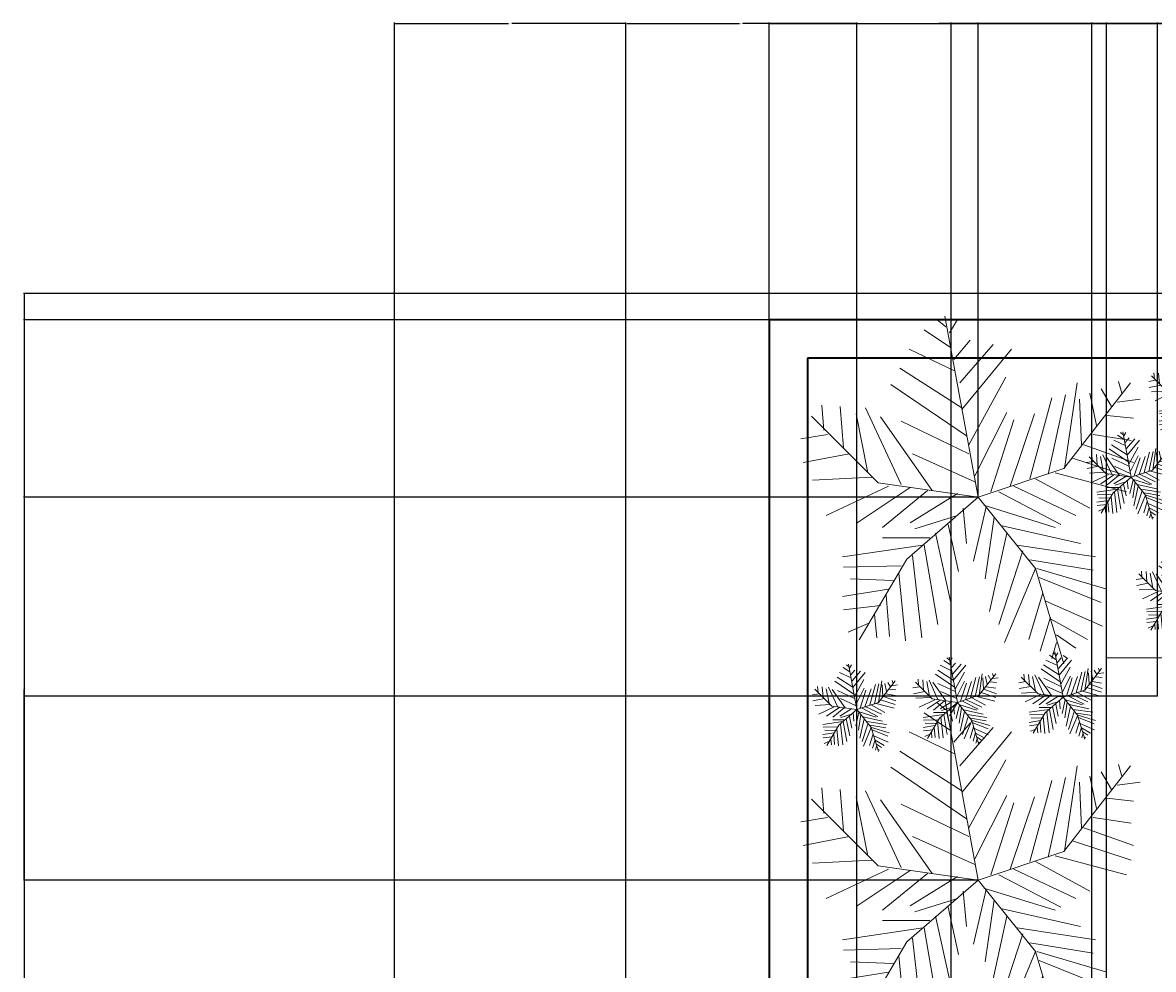
# Model space of a CAD drawing. Units: inches. Extents: x 818 to 1898, y 976 to 2364.
# Tile 61 of 96: x 818 to 1083, y 2142 to 2364. Entities that reach past the tile are written whole.
import ezdxf

# ---------------------------------------------------------------- set-up
doc = ezdxf.new("R2010")
doc.units = ezdxf.units.IN
doc.header["$LTSCALE"] = 5
doc.header["$MEASUREMENT"] = 0
for name, color, linetype, lineweight in [('A-ANNO-DIMS', 2, 'Continuous', 18), ('C-PROP', 7, 'Continuous', 35), ('L-PLNT-BEDS', 94, 'Continuous', 18)]:
    doc.layers.add(name, color=color, linetype=linetype, lineweight=lineweight)
doc.layers.add('L-PLNT', color=116, linetype='Continuous', lineweight=13, true_color=0x136734)
doc.styles.get("Standard").update_dxf_attribs({"font": 'arial.ttf'})
doc.dimstyles.get("Standard").update_dxf_attribs({"dimtxt": 0.18, "dimasz": 0.18, "dimexe": 0.18, "dimexo": 0.0625, "dimgap": 0.09, "dimtad": 0, "dimtih": 1, "dimtoh": 1, "dimdec": 4, "dimzin": 0, "dimdsep": 46, "dimtxsty": 'Standard', "dimcen": 0.09, "dimadec": 0, "dimazin": 0, "dimtfac": 1, "dimtdec": 4, "dimtofl": 0, "dimtmove": 0, "dimatfit": 3, "dimfxl": 1, "dimtolj": 1, "dimtzin": 0, "dimarcsym": 0})

# ---------------------------------------------------------------- blocks, each defined once
blk = doc.blocks.new('SHRUB-ACCENT')
for p, q in [((8.8, 18.63), (7.25, 19.67)), ((8.53, 19.84), (7.99, 20.28)), ((10.44, 9.82), (8.47, 20.47)), ((8.74, 19.5), (9.21, 20.28)), ((9.01, 17.93), (9.96, 19.06)), ((9.35, 16.54), (11.31, 18.8)), ((9.75, 13.42), (5.28, 16.46)), ((9.48, 15.07), (5.82, 17.41)), ((9.08, 17.24), (6.37, 18.54)), ((9.48, 14.98), (12.39, 18.54)), ((9.89, 12.9), (12.06, 16.89)), ((15.49, 11.5), (19.41, 16.55)), ((15.51, 11.51), (16.25, 16.54)), ((17, 15.94), (17.41, 14.03)), ((17.68, 16.2), (18.29, 15.16)), ((18.69, 16.63), (18.9, 15.94)), ((1.56, 13.51), (0, 13.25)), ((4.55, 10.66), (0.62, 14.58)), ((1.35, 13.77), (1.22, 15.24)), ((2.3, 15.16), (2.51, 12.72)), ((3.25, 14.72), (3.93, 11.25)), ((3.79, 15.07), (5.89, 10.55)), ((7.72, 10.21), (4.67, 14.55)), ((5.89, 14.29), (9.89, 12.38)), ((10.23, 11.07), (12.12, 14.81)), ((11.17, 10.12), (12.53, 14.37)), ((12.33, 10.47), (13.75, 14.72)), ((13.48, 10.9), (14.76, 15.68)), ((14.56, 11.16), (15.58, 15.85)), ((16.39, 15.59), (16.53, 12.9)), ((17.2, 13.51), (19.44, 13.16)), ((18.02, 14.63), (19.57, 14.46)), ((18.62, 15.42), (19.98, 15.59)), ((2.84, 12.38), (0.14, 11.86)), ((4.2, 10.99), (0.68, 10.81)), ((10.44, 9.82), (4.55, 10.66)), ((6.57, 12.38), (10.23, 10.73)), ((10.44, 9.82), (15.49, 11.5)), ((13.82, 10.9), (17, 9.16)), ((14.97, 11.25), (19.17, 10.12)), ((15.98, 12.12), (19.44, 10.99)), ((16.66, 12.9), (19.57, 11.86)), ((5.15, 10.47), (1.49, 8.73)), ((6.43, 10.38), (3.32, 8.3)), ((7.45, 10.21), (4.81, 8.04)), ((10.44, 9.82), (6.23, 6.17)), ((9.21, 10.03), (6.43, 8.3)), ((9.21, 8.73), (6.7, 7.95)), ((8.67, 8.21), (9.28, 5.43)), ((9.55, 9.16), (9.75, 7.08)), ((10.9, 9.25), (10.16, 6.04)), ((10.44, 9.82), (13.8, 5.61)), ((10.77, 9.34), (14.97, 8.04)), ((11.38, 8.64), (10.84, 5)), ((11.65, 10.12), (15.31, 8.21)), ((11.85, 8.12), (16.46, 7.08)), ((12.53, 10.47), (16.19, 8.73)), ((7.18, 6.99), (2.44, 6.3)), ((5.89, 5.78), (2.51, 5.69)), ((6.23, 6.17), (3.43, 1.4)), ((7.59, 7.43), (4.81, 7.43)), ((5.76, 5.34), (6.16, 1.35)), ((6.57, 6.39), (7.11, 1.52)), ((7.25, 6.99), (8.06, 2.31)), ((7.92, 7.69), (8.8, 3.69)), ((12.12, 7.69), (11.11, 3.09)), ((13.07, 6.65), (11.65, 2.31)), ((13.82, 5.6), (11.99, 1.26)), ((12.73, 6.99), (17.34, 6.3)), ((13.48, 6.13), (17.2, 5.52)), ((13.8, 5.61), (15.49, 0)), ((13.88, 5.6), (18.02, 4.39)), ((5.15, 4.39), (2.44, 3.95)), ((4.67, 3.43), (2.51, 3.17)), ((5.42, 4.91), (2.91, 5)), ((4.33, 2.91), (4.47, 1.52)), ((5.01, 4.04), (5.21, 1.61)), ((14.22, 4.13), (13.41, 1.44)), ((14.02, 5.08), (17.68, 3.61)), ((14.7, 2.74), (14.09, 0.74)), ((14.43, 3.69), (17.74, 2.22)), ((14.7, 2.65), (16.86, 1.44)), ((4, 2.39), (2.78, 1.87)), ((15.04, 1.26), (14.76, 0.31)), ((15.04, 1.7), (16.19, 0.92)), ((15.44, 0.48), (15.71, 0.31))]:
    blk.add_line(p, q)
blk = doc.blocks.new('PALM-BORDER')
for p, q in [((33.95, 78.95), (31.8, 80.68)), ((41.53, 39.05), (33.72, 81.45)), ((34.76, 77.57), (36.65, 80.68)), ((35.03, 74.11), (28.83, 78.26)), ((35.84, 71.35), (39.61, 75.84)), ((37.18, 65.82), (45, 74.8)), ((36.11, 68.59), (25.33, 73.77)), ((37.72, 59.6), (49.31, 73.77)), ((37.72, 59.95), (23.17, 69.28)), ((39.34, 51.31), (47.96, 67.2)), ((38.8, 53.39), (21.02, 65.48)), ((61.61, 45.75), (77.23, 65.83)), ((61.71, 45.79), (64.67, 65.82)), ((70.33, 64.44), (72.75, 60.3)), ((74.37, 66.17), (75.18, 63.4)), ((53.62, 43.37), (58.74, 62.37)), ((57.93, 44.41), (61.97, 63.06)), ((65.21, 62.02), (65.75, 51.31)), ((67.63, 63.4), (69.25, 55.81)), ((74.1, 61.33), (79.49, 62.02)), ((5.39, 54.77), (4.85, 60.64)), ((9.16, 60.3), (9.97, 50.62)), ((12.93, 58.57), (15.63, 44.75)), ((15.09, 59.95), (23.44, 41.99)), ((40.69, 44.06), (48.23, 58.91)), ((49.04, 41.64), (54.7, 58.57)), ((18.1, 42.4), (2.48, 58.02)), ((30.72, 40.61), (18.59, 57.88)), ((23.44, 56.84), (39.34, 49.24)), ((44.46, 40.26), (49.85, 57.19)), ((71.68, 58.22), (77.87, 57.53)), ((6.2, 53.73), (0, 52.7)), ((68.44, 53.73), (77.33, 52.35)), ((66.29, 51.31), (77.87, 47.17)), ((11.32, 49.24), (0.54, 47.17)), ((26.14, 49.24), (40.69, 42.68)), ((63.59, 48.21), (77.33, 43.71)), ((41.53, 39.05), (61.61, 45.75)), ((16.71, 43.71), (2.69, 43.02)), ((41.53, 39.05), (18.1, 42.4)), ((54.97, 43.37), (67.63, 36.46)), ((59.55, 44.75), (76.26, 40.26)), ((20.48, 41.64), (5.93, 34.73)), ((25.6, 41.3), (13.2, 33.01)), ((29.64, 40.61), (19.13, 31.97)), ((36.65, 39.91), (25.6, 33.01)), ((46.35, 40.26), (60.9, 32.66)), ((49.85, 41.64), (64.4, 34.73)), ((41.53, 39.05), (24.79, 24.55)), ((41.53, 39.05), (54.92, 22.32)), ((42.84, 37.15), (59.55, 31.97)), ((36.65, 34.73), (26.68, 31.62)), ((37.99, 36.46), (38.8, 28.17)), ((43.38, 36.81), (40.42, 24.02)), ((34.49, 32.66), (36.92, 21.61)), ((45.27, 34.39), (43.11, 19.88)), ((47.15, 32.32), (65.48, 28.17)), ((30.18, 29.55), (19.13, 29.55)), ((31.53, 30.59), (35.03, 14.7)), ((48.23, 30.59), (44.19, 12.28)), ((28.56, 27.82), (9.7, 25.06)), ((28.83, 27.82), (32.07, 9.17)), ((50.66, 27.82), (68.98, 25.06)), ((24.79, 24.55), (13.63, 5.58)), ((26.14, 25.41), (28.29, 6.06)), ((52, 26.44), (46.35, 9.17)), ((53.62, 24.37), (68.44, 21.95)), ((23.44, 22.99), (9.97, 22.64)), ((22.9, 21.26), (24.52, 5.37)), ((54.97, 22.3), (47.69, 5.02)), ((54.92, 22.32), (61.61, 0)), ((55.24, 22.3), (71.68, 17.46)), ((21.56, 19.53), (11.59, 19.88)), ((55.78, 20.22), (70.33, 14.35)), ((20.48, 17.46), (9.7, 15.73)), ((19.94, 16.08), (20.75, 6.41)), ((56.59, 16.42), (53.35, 5.72)), ((18.59, 13.66), (9.97, 12.62)), ((57.39, 14.7), (70.6, 8.83)), ((17.24, 11.59), (17.78, 6.06)), ((58.47, 10.9), (56.05, 2.95)), ((15.9, 9.52), (11.05, 7.44)), ((58.47, 10.55), (67.09, 5.72)), ((59.82, 6.75), (64.4, 3.64)), ((59.82, 5.02), (58.74, 1.22)), ((61.44, 1.92), (62.51, 1.22))]:
    blk.add_line(p, q)
blk = doc.blocks.new('*D57')
at = {"layer": 'A-ANNO-DIMS', "color": 0, "lineweight": -2, "ltscale": 5, "transparency": 16777216}
for p, q in [((992.73, 2294.28), (992.73, 2363.87)), ((992.91, 2363.69), (1395.43, 2363.69)), ((1798.54, 2363.69), (1396.01, 2363.69)), ((1798.72, 2294.28), (1798.72, 2363.87))]:
    blk.add_line(p, q, dxfattribs=at)
at = {"layer": 'A-ANNO-DIMS', "color": 0, "ltscale": 5, "transparency": 16777216}
for points in [[(992.91, 2363.72), (992.91, 2363.66), (992.73, 2363.69)], [(1798.54, 2363.72), (1798.54, 2363.66), (1798.72, 2363.69)]]:
    blk.add_solid(points, dxfattribs=at)
at = {"layer": 'Defpoints', "color": 0, "ltscale": 5, "transparency": 16777216}
for p in [(1798.72, 2363.69), (992.73, 2294.22), (1798.72, 2294.22)]:
    blk.add_point(p, dxfattribs=at)
at = {"layer": 'A-ANNO-DIMS', "color": 0, "ltscale": 5, "transparency": 16777216, "insert": (1395.72, 2363.69), "char_height": 0.18, "attachment_point": 5}
blk.add_mtext('\\A1;806', dxfattribs=at)
blk = doc.blocks.new('*D59')
at = {"layer": 'A-ANNO-DIMS', "color": 0, "lineweight": -2, "ltscale": 5, "transparency": 16777216}
for p, q in [((1251.64, 2300.39), (818.03, 2300.39)), ((818.21, 2300.21), (818.21, 1669.95)), ((818.21, 1039.32), (818.21, 1669.59)), ((896.05, 1039.14), (818.03, 1039.14))]:
    blk.add_line(p, q, dxfattribs=at)
at = {"layer": 'A-ANNO-DIMS', "color": 0, "ltscale": 5, "transparency": 16777216}
for points in [[(818.18, 2300.21), (818.24, 2300.21), (818.21, 2300.39)], [(818.18, 1039.32), (818.24, 1039.32), (818.21, 1039.14)]]:
    blk.add_solid(points, dxfattribs=at)
at = {"layer": 'Defpoints', "color": 0, "ltscale": 5, "transparency": 16777216}
for p in [(818.21, 2300.39), (1251.71, 2300.39), (896.11, 1039.14)]:
    blk.add_point(p, dxfattribs=at)
at = {"layer": 'A-ANNO-DIMS', "color": 0, "ltscale": 5, "transparency": 16777216, "insert": (818.21, 1669.77), "char_height": 0.18, "attachment_point": 5}
blk.add_mtext('\\A1;1261.2', dxfattribs=at)
blk = doc.blocks.new('*D60')
at = {"layer": 'A-ANNO-DIMS', "color": 0, "lineweight": -2, "ltscale": 5, "transparency": 16777216}
for p, q in [((992.66, 2294.22), (818.03, 2294.22)), ((818.21, 2294.04), (818.21, 1748.77)), ((818.21, 1203.14), (818.21, 1748.41)), ((992.66, 1202.96), (818.03, 1202.96))]:
    blk.add_line(p, q, dxfattribs=at)
at = {"layer": 'A-ANNO-DIMS', "color": 0, "ltscale": 5, "transparency": 16777216}
for points in [[(818.18, 2294.04), (818.24, 2294.04), (818.21, 2294.22)], [(818.18, 1203.14), (818.24, 1203.14), (818.21, 1202.96)]]:
    blk.add_solid(points, dxfattribs=at)
at = {"layer": 'Defpoints', "color": 0, "ltscale": 5, "transparency": 16777216}
for p in [(818.21, 2294.22), (992.73, 2294.22), (992.73, 1202.96)]:
    blk.add_point(p, dxfattribs=at)
at = {"layer": 'A-ANNO-DIMS', "color": 0, "ltscale": 5, "transparency": 16777216, "insert": (818.21, 1748.59), "char_height": 0.18, "attachment_point": 5}
blk.add_mtext('\\A1;1091.3', dxfattribs=at)
blk = doc.blocks.new('*D61')
at = {"layer": 'A-ANNO-DIMS', "color": 0, "lineweight": -2, "ltscale": 5, "transparency": 16777216}
for p, q in [((1071.73, 1203.03), (1071.73, 2363.87)), ((1071.91, 2363.69), (1250.94, 2363.69)), ((1430.55, 2363.69), (1251.51, 2363.69)), ((1430.73, 1203.03), (1430.73, 2363.87))]:
    blk.add_line(p, q, dxfattribs=at)
at = {"layer": 'A-ANNO-DIMS', "color": 0, "ltscale": 5, "transparency": 16777216}
for points in [[(1071.91, 2363.72), (1071.91, 2363.66), (1071.73, 2363.69)], [(1430.55, 2363.72), (1430.55, 2363.66), (1430.73, 2363.69)]]:
    blk.add_solid(points, dxfattribs=at)
at = {"layer": 'Defpoints', "color": 0, "ltscale": 5, "transparency": 16777216}
for p in [(1430.73, 2363.69), (1071.73, 1202.96), (1430.73, 1202.96)]:
    blk.add_point(p, dxfattribs=at)
at = {"layer": 'A-ANNO-DIMS', "color": 0, "ltscale": 5, "transparency": 16777216, "insert": (1251.23, 2363.69), "char_height": 0.18, "attachment_point": 5}
blk.add_mtext('\\A1;359', dxfattribs=at)
blk = doc.blocks.new('*D67')
at = {"layer": 'A-ANNO-DIMS', "color": 0, "lineweight": -2, "ltscale": 5, "transparency": 16777216}
for p, q in [((1083.66, 2205.97), (818.03, 2205.97)), ((818.21, 2205.79), (818.21, 2129.71)), ((818.21, 2053.26), (818.21, 2129.34)), ((1083.66, 2053.08), (818.03, 2053.08))]:
    blk.add_line(p, q, dxfattribs=at)
at = {"layer": 'A-ANNO-DIMS', "color": 0, "ltscale": 5, "transparency": 16777216}
for points in [[(818.18, 2205.79), (818.24, 2205.79), (818.21, 2205.97)], [(818.18, 2053.26), (818.24, 2053.26), (818.21, 2053.08)]]:
    blk.add_solid(points, dxfattribs=at)
at = {"layer": 'Defpoints', "color": 0, "ltscale": 5, "transparency": 16777216}
for p in [(818.21, 2205.97), (1083.73, 2205.97), (1083.73, 2053.08)]:
    blk.add_point(p, dxfattribs=at)
at = {"layer": 'A-ANNO-DIMS', "color": 0, "ltscale": 5, "transparency": 16777216, "insert": (818.21, 2129.52), "char_height": 0.18, "attachment_point": 5}
blk.add_mtext('\\A1;152.9', dxfattribs=at)
blk = doc.blocks.new('*D79')
at = {"layer": 'A-ANNO-DIMS', "color": 0, "lineweight": -2, "ltscale": 5, "transparency": 16777216}
for p, q in [((992.73, 1203.03), (992.73, 2363.87)), ((992.91, 2363.69), (1032.01, 2363.69)), ((1071.55, 2363.69), (1032.44, 2363.69)), ((1071.73, 1203.03), (1071.73, 2363.87))]:
    blk.add_line(p, q, dxfattribs=at)
at = {"layer": 'A-ANNO-DIMS', "color": 0, "ltscale": 5, "transparency": 16777216}
for points in [[(992.91, 2363.72), (992.91, 2363.66), (992.73, 2363.69)], [(1071.55, 2363.72), (1071.55, 2363.66), (1071.73, 2363.69)]]:
    blk.add_solid(points, dxfattribs=at)
at = {"layer": 'Defpoints', "color": 0, "ltscale": 5, "transparency": 16777216}
for p in [(1071.73, 2363.69), (992.73, 1202.96), (1071.73, 1202.96)]:
    blk.add_point(p, dxfattribs=at)
at = {"layer": 'A-ANNO-DIMS', "color": 0, "ltscale": 5, "transparency": 16777216, "insert": (1032.23, 2363.69), "char_height": 0.18, "attachment_point": 5}
blk.add_mtext('\\A1;79', dxfattribs=at)
blk = doc.blocks.new('*D87')
at = {"layer": 'A-ANNO-DIMS', "color": 0, "lineweight": -2, "ltscale": 5, "transparency": 16777216}
for p, q in [((992.73, 2294.28), (992.73, 2363.87)), ((992.91, 2363.69), (1038.02, 2363.69)), ((1083.55, 2363.69), (1038.43, 2363.69)), ((1083.73, 2206.03), (1083.73, 2363.87))]:
    blk.add_line(p, q, dxfattribs=at)
at = {"layer": 'A-ANNO-DIMS', "color": 0, "ltscale": 5, "transparency": 16777216}
for points in [[(992.91, 2363.72), (992.91, 2363.66), (992.73, 2363.69)], [(1083.55, 2363.72), (1083.55, 2363.66), (1083.73, 2363.69)]]:
    blk.add_solid(points, dxfattribs=at)
at = {"layer": 'Defpoints', "color": 0, "ltscale": 5, "transparency": 16777216}
for p in [(1083.73, 2363.69), (992.73, 2294.22), (1083.73, 2205.97)]:
    blk.add_point(p, dxfattribs=at)
at = {"layer": 'A-ANNO-DIMS', "color": 0, "ltscale": 5, "transparency": 16777216, "insert": (1038.23, 2363.69), "char_height": 0.18, "attachment_point": 5}
blk.add_mtext('\\A1;91', dxfattribs=at)
blk = doc.blocks.new('*D90')
at = {"layer": 'A-ANNO-DIMS', "color": 0, "lineweight": -2, "ltscale": 5, "transparency": 16777216}
for p, q in [((904.95, 1071.12), (904.95, 2363.87)), ((905.13, 2363.69), (931.67, 2363.69)), ((958.99, 2363.69), (932.45, 2363.69)), ((959.17, 1071.12), (959.17, 2363.87))]:
    blk.add_line(p, q, dxfattribs=at)
at = {"layer": 'A-ANNO-DIMS', "color": 0, "ltscale": 5, "transparency": 16777216}
for points in [[(905.13, 2363.72), (905.13, 2363.66), (904.95, 2363.69)], [(958.99, 2363.72), (958.99, 2363.66), (959.17, 2363.69)]]:
    blk.add_solid(points, dxfattribs=at)
at = {"layer": 'Defpoints', "color": 0, "ltscale": 5, "transparency": 16777216}
for p in [(959.17, 2363.69), (904.95, 1071.06), (959.17, 1071.06)]:
    blk.add_point(p, dxfattribs=at)
at = {"layer": 'A-ANNO-DIMS', "color": 0, "ltscale": 5, "transparency": 16777216, "insert": (932.06, 2363.69), "char_height": 0.18, "attachment_point": 5}
blk.add_mtext('\\A1;54.22', dxfattribs=at)
blk = doc.blocks.new('*D91')
at = {"layer": 'A-ANNO-DIMS', "color": 0, "lineweight": -2, "ltscale": 5, "transparency": 16777216}
for p, q in [((959.17, 1071.12), (959.17, 2363.87)), ((959.35, 2363.69), (985.8, 2363.69)), ((1013.04, 2363.69), (986.59, 2363.69)), ((1013.22, 1071.12), (1013.22, 2363.87))]:
    blk.add_line(p, q, dxfattribs=at)
at = {"layer": 'A-ANNO-DIMS', "color": 0, "ltscale": 5, "transparency": 16777216}
for points in [[(959.35, 2363.72), (959.35, 2363.66), (959.17, 2363.69)], [(1013.04, 2363.72), (1013.04, 2363.66), (1013.22, 2363.69)]]:
    blk.add_solid(points, dxfattribs=at)
at = {"layer": 'Defpoints', "color": 0, "ltscale": 5, "transparency": 16777216}
for p in [(1013.22, 2363.69), (959.17, 1071.06), (1013.22, 1071.06)]:
    blk.add_point(p, dxfattribs=at)
at = {"layer": 'A-ANNO-DIMS', "color": 0, "ltscale": 5, "transparency": 16777216, "insert": (986.2, 2363.69), "char_height": 0.18, "attachment_point": 5}
blk.add_mtext('\\A1;54.04', dxfattribs=at)
blk = doc.blocks.new('*D92')
at = {"layer": 'A-ANNO-DIMS', "color": 0, "lineweight": -2, "ltscale": 5, "transparency": 16777216}
for p, q in [((1013.22, 1071.12), (1013.22, 2363.87)), ((1013.4, 2363.69), (1040.38, 2363.69)), ((1068.16, 2363.69), (1041.17, 2363.69)), ((1068.34, 1071.12), (1068.34, 2363.87))]:
    blk.add_line(p, q, dxfattribs=at)
at = {"layer": 'A-ANNO-DIMS', "color": 0, "ltscale": 5, "transparency": 16777216}
for points in [[(1013.4, 2363.72), (1013.4, 2363.66), (1013.22, 2363.69)], [(1068.16, 2363.72), (1068.16, 2363.66), (1068.34, 2363.69)]]:
    blk.add_solid(points, dxfattribs=at)
at = {"layer": 'Defpoints', "color": 0, "ltscale": 5, "transparency": 16777216}
for p in [(1068.34, 2363.69), (1013.22, 1071.06), (1068.34, 1071.06)]:
    blk.add_point(p, dxfattribs=at)
at = {"layer": 'A-ANNO-DIMS', "color": 0, "ltscale": 5, "transparency": 16777216, "insert": (1040.78, 2363.69), "char_height": 0.18, "attachment_point": 5}
blk.add_mtext('\\A1;55.12', dxfattribs=at)
blk = doc.blocks.new('*D93')
at = {"layer": 'A-ANNO-DIMS', "color": 0, "lineweight": -2, "ltscale": 5, "transparency": 16777216}
for p, q in [((1068.34, 1071.12), (1068.34, 2363.87)), ((1068.52, 2363.69), (1094.16, 2363.69)), ((1120.58, 2363.69), (1094.94, 2363.69)), ((1120.76, 1071.12), (1120.76, 2363.87))]:
    blk.add_line(p, q, dxfattribs=at)
at = {"layer": 'A-ANNO-DIMS', "color": 0, "ltscale": 5, "transparency": 16777216}
for points in [[(1068.52, 2363.72), (1068.52, 2363.66), (1068.34, 2363.69)], [(1120.58, 2363.72), (1120.58, 2363.66), (1120.76, 2363.69)]]:
    blk.add_solid(points, dxfattribs=at)
at = {"layer": 'Defpoints', "color": 0, "ltscale": 5, "transparency": 16777216}
for p in [(1120.76, 2363.69), (1068.34, 1071.06), (1120.76, 1071.06)]:
    blk.add_point(p, dxfattribs=at)
at = {"layer": 'A-ANNO-DIMS', "color": 0, "ltscale": 5, "transparency": 16777216, "insert": (1094.55, 2363.69), "char_height": 0.18, "attachment_point": 5}
blk.add_mtext('\\A1;52.42', dxfattribs=at)
blk = doc.blocks.new('*D126')
at = {"layer": 'A-ANNO-DIMS', "color": 0, "lineweight": -2, "ltscale": 5, "transparency": 16777216}
for p, q in [((1035.38, 1252.09), (1035.38, 2363.87)), ((1035.56, 2363.69), (1075.41, 2363.69)), ((1116.01, 2363.69), (1076.16, 2363.69)), ((1116.19, 1236.03), (1116.19, 2363.87))]:
    blk.add_line(p, q, dxfattribs=at)
at = {"layer": 'A-ANNO-DIMS', "color": 0, "ltscale": 5, "transparency": 16777216}
for points in [[(1035.56, 2363.72), (1035.56, 2363.66), (1035.38, 2363.69)], [(1116.01, 2363.72), (1116.01, 2363.66), (1116.19, 2363.69)]]:
    blk.add_solid(points, dxfattribs=at)
at = {"layer": 'Defpoints', "color": 0, "ltscale": 5, "transparency": 16777216}
for p in [(1035.38, 2363.69), (1035.38, 1252.02), (1116.19, 1235.96)]:
    blk.add_point(p, dxfattribs=at)
at = {"layer": 'A-ANNO-DIMS', "color": 0, "ltscale": 5, "transparency": 16777216, "insert": (1075.78, 2363.69), "char_height": 0.18, "attachment_point": 5}
blk.add_mtext('\\A1;80.81', dxfattribs=at)
blk = doc.blocks.new('*D133')
at = {"layer": 'A-ANNO-DIMS', "color": 0, "lineweight": -2, "ltscale": 5, "transparency": 16777216}
for p, q in [((1041.64, 2162.89), (818.03, 2162.89)), ((818.21, 2162.71), (818.21, 2101.01)), ((818.21, 2038.94), (818.21, 2100.64)), ((1043.71, 2038.76), (818.03, 2038.76))]:
    blk.add_line(p, q, dxfattribs=at)
at = {"layer": 'A-ANNO-DIMS', "color": 0, "ltscale": 5, "transparency": 16777216}
for points in [[(818.18, 2162.71), (818.24, 2162.71), (818.21, 2162.89)], [(818.18, 2038.94), (818.24, 2038.94), (818.21, 2038.76)]]:
    blk.add_solid(points, dxfattribs=at)
at = {"layer": 'Defpoints', "color": 0, "ltscale": 5, "transparency": 16777216}
for p in [(818.21, 2162.89), (1041.7, 2162.89), (1043.77, 2038.76)]:
    blk.add_point(p, dxfattribs=at)
at = {"layer": 'A-ANNO-DIMS', "color": 0, "ltscale": 5, "transparency": 16777216, "insert": (818.21, 2100.82), "char_height": 0.18, "attachment_point": 5}
blk.add_mtext('\\A1;124.13', dxfattribs=at)
blk = doc.blocks.new('*D134')
at = {"layer": 'A-ANNO-DIMS', "color": 0, "lineweight": -2, "ltscale": 5, "transparency": 16777216}
for p, q in [((1041.64, 2252.64), (818.03, 2252.64)), ((818.21, 2252.46), (818.21, 2207.95)), ((818.21, 2163.07), (818.21, 2207.58)), ((1041.64, 2162.89), (818.03, 2162.89))]:
    blk.add_line(p, q, dxfattribs=at)
at = {"layer": 'A-ANNO-DIMS', "color": 0, "ltscale": 5, "transparency": 16777216}
for points in [[(818.18, 2252.46), (818.24, 2252.46), (818.21, 2252.64)], [(818.18, 2163.07), (818.24, 2163.07), (818.21, 2162.89)]]:
    blk.add_solid(points, dxfattribs=at)
at = {"layer": 'Defpoints', "color": 0, "ltscale": 5, "transparency": 16777216}
for p in [(818.21, 2252.64), (1041.7, 2252.64), (1041.7, 2162.89)]:
    blk.add_point(p, dxfattribs=at)
at = {"layer": 'A-ANNO-DIMS', "color": 0, "ltscale": 5, "transparency": 16777216, "insert": (818.21, 2207.77), "char_height": 0.18, "attachment_point": 5}
blk.add_mtext('\\A1;89.75', dxfattribs=at)
blk = doc.blocks.new('*D135')
at = {"layer": 'A-ANNO-DIMS', "color": 0, "lineweight": -2, "ltscale": 5, "transparency": 16777216}
for p, q in [((1041.7, 2252.7), (1041.7, 2363.87)), ((1041.88, 2363.69), (1096.11, 2363.69)), ((1151.25, 2363.69), (1097.02, 2363.69)), ((1151.43, 2252.7), (1151.43, 2363.87))]:
    blk.add_line(p, q, dxfattribs=at)
at = {"layer": 'A-ANNO-DIMS', "color": 0, "ltscale": 5, "transparency": 16777216}
for points in [[(1041.88, 2363.72), (1041.88, 2363.66), (1041.7, 2363.69)], [(1151.25, 2363.72), (1151.25, 2363.66), (1151.43, 2363.69)]]:
    blk.add_solid(points, dxfattribs=at)
at = {"layer": 'Defpoints', "color": 0, "ltscale": 5, "transparency": 16777216}
for p in [(1151.43, 2363.69), (1041.7, 2252.64), (1151.43, 2252.64)]:
    blk.add_point(p, dxfattribs=at)
at = {"layer": 'A-ANNO-DIMS', "color": 0, "ltscale": 5, "transparency": 16777216, "insert": (1096.56, 2363.69), "char_height": 0.18, "attachment_point": 5}
blk.add_mtext('\\A1;109.72', dxfattribs=at)

msp = doc.modelspace()

# ---------------------------------------------------------------- linework, layer by layer
at = {"layer": 'C-PROP', "ltscale": 5}
for p, q in [((1798.7173, 2294.2171), (992.7251, 2294.2171)), ((1789.7173, 2285.2171), (1001.7252, 2285.2171))]:
    msp.add_line(p, q, dxfattribs=at)
at = {"layer": 'C-PROP'}
for p, q in [((992.7251, 2294.2171), (992.7251, 1202.9642)), ((1001.7252, 2285.2171), (1001.7252, 1211.9642))]:
    msp.add_line(p, q, dxfattribs=at)
at = {"layer": 'L-PLNT-BEDS'}
msp.add_line((1071.7251, 2214.9709), (1071.7251, 1202.9642), dxfattribs=at)
at = {"layer": 'L-PLNT-BEDS', "ltscale": 5}
msp.add_line((1789.7173, 2214.9709), (1071.7251, 2214.9709), dxfattribs=at)

# ---------------------------------------------------------------- block references
at = {"layer": 'L-PLNT'}
for name, p in [('PALM-BORDER', (1000.173, 2213.5896)), ('SHRUB-ACCENT', (1081.633, 2266.5141)), ('SHRUB-ACCENT', (1067.0685, 2247.4883)), ('SHRUB-ACCENT', (1078.7017, 2220.0709)), ('SHRUB-ACCENT', (1026.3812, 2194.7004)), ('SHRUB-ACCENT', (1051.1707, 2195.9064)), ('SHRUB-ACCENT', (1002.8335, 2193.0293)), ('PALM-BORDER', (1000.173, 2123.8387))]:
    msp.add_blockref(name, p, dxfattribs=at)

# ---------------------------------------------------------------- dimensions: what is measured, and where the dimension line sits
at = {"layer": 'A-ANNO-DIMS', "ltscale": 5}
for base, p1, p2, override, picture, middle in [((959.1737, 2363.6929), (904.9504, 1071.0552), (959.1737, 1071.0552), {"dimdec": 2, "dimlfac": 1, "dimrnd": 0, "dimzin": 0, "dimdsep": 46, "dimlunit": 2}, '*D90', (932.062, 2363.6929)), ((1013.2176, 2363.6929), (959.1737, 1071.0552), (1013.2176, 1071.0552), {"dimdec": 2, "dimlfac": 1, "dimrnd": 0, "dimzin": 0, "dimdsep": 46, "dimlunit": 2}, '*D91', (986.1956, 2363.6929)), ((1798.7173, 2363.6929), (992.7251, 2294.2171), (1798.7173, 2294.2171), {"dimdec": 0, "dimlfac": 1, "dimrnd": 0, "dimzin": 0, "dimdsep": 46, "dimlunit": 2}, '*D57', (1395.7212, 2363.6929)), ((1071.7251, 2363.6929), (992.7251, 1202.9642), (1071.7251, 1202.9642), {"dimdec": 0, "dimlfac": 1, "dimrnd": 0, "dimzin": 0, "dimdsep": 46, "dimlunit": 2}, '*D79', (1032.2251, 2363.6929)), ((1083.7251, 2363.6929), (992.7251, 2294.2171), (1083.7251, 2205.9709), {"dimdec": 0, "dimlfac": 1, "dimrnd": 0, "dimzin": 0, "dimdsep": 46, "dimlunit": 2}, '*D87', (1038.2251, 2363.6929)), ((1068.3377, 2363.6929), (1013.2176, 1071.0552), (1068.3377, 1071.0552), {"dimdec": 2, "dimlfac": 1, "dimrnd": 0, "dimzin": 0, "dimdsep": 46, "dimlunit": 2}, '*D92', (1040.7776, 2363.6929)), ((1035.3768, 2363.6929), (1116.1882, 1235.9642), (1035.3768, 1252.0242), {"dimdec": 2, "dimlfac": 1, "dimrnd": 0, "dimzin": 0, "dimdsep": 46, "dimlunit": 2}, '*D126', (1075.7825, 2363.6929)), ((1151.4251, 2363.6929), (1041.7008, 2252.6408), (1151.4251, 2252.6408), {"dimdec": 2, "dimlfac": 1, "dimrnd": 0, "dimzin": 0, "dimdsep": 46, "dimlunit": 2}, '*D135', (1096.5629, 2363.6929)), ((1120.7618, 2363.6929), (1068.3377, 1071.0552), (1120.7618, 1071.0552), {"dimdec": 2, "dimlfac": 1, "dimrnd": 0, "dimzin": 0, "dimdsep": 46, "dimlunit": 2}, '*D93', (1094.5497, 2363.6929)), ((1430.7251, 2363.6929), (1071.7251, 1202.9642), (1430.7251, 1202.9642), {"dimdec": 0, "dimlfac": 1, "dimrnd": 0, "dimzin": 0, "dimdsep": 46, "dimlunit": 2}, '*D61', (1251.2251, 2363.6929))]:
    dim = msp.add_linear_dim(base=base, p1=p1, p2=p2, dimstyle='Standard', override=override, dxfattribs=at)
    dim.commit()
    dim.dimension.update_dxf_attribs({"geometry": picture, "text_midpoint": middle})
for base, p1, p2, override, picture, middle in [((818.2059, 2300.3929), (896.1138, 1039.1433), (1251.7057, 2300.3929), {"dimdec": 1, "dimlfac": 1, "dimrnd": 0, "dimzin": 0, "dimdsep": 46, "dimlunit": 2}, '*D59', (818.2059, 1669.7681)), ((818.2059, 2294.2171), (992.7251, 1202.9642), (992.7251, 2294.2171), {"dimdec": 1, "dimlfac": 1, "dimrnd": 0, "dimzin": 0, "dimdsep": 46, "dimlunit": 2}, '*D60', (818.2059, 1748.5907)), ((818.2059, 2252.6408), (1041.7008, 2162.8898), (1041.7008, 2252.6408), {"dimdec": 2, "dimlfac": 1, "dimrnd": 0, "dimzin": 0, "dimdsep": 46, "dimlunit": 2}, '*D134', (818.2059, 2207.7653)), ((818.2059, 2205.9709), (1083.7251, 2053.0782), (1083.7251, 2205.9709), {"dimdec": 1, "dimlfac": 1, "dimrnd": 0, "dimzin": 0, "dimdsep": 46, "dimlunit": 2}, '*D67', (818.2059, 2129.5246)), ((818.2059, 2162.8898), (1043.7685, 2038.7583), (1041.7008, 2162.8898), {"dimdec": 2, "dimlfac": 1, "dimrnd": 0, "dimzin": 0, "dimdsep": 46, "dimlunit": 2}, '*D133', (818.2059, 2100.824))]:
    dim = msp.add_linear_dim(base=base, p1=p1, p2=p2, angle=90, dimstyle='Standard', override=override, dxfattribs=at)
    dim.commit()
    dim.dimension.update_dxf_attribs({"geometry": picture, "text_midpoint": middle})

doc.saveas('drawing.dxf')
